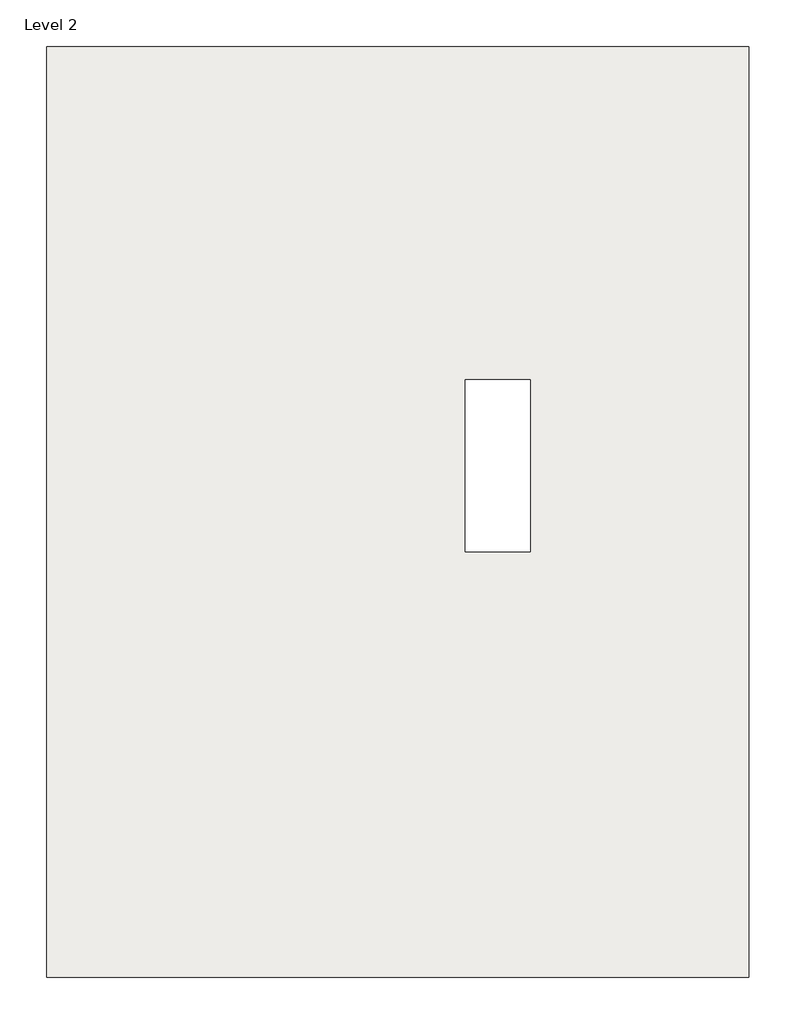
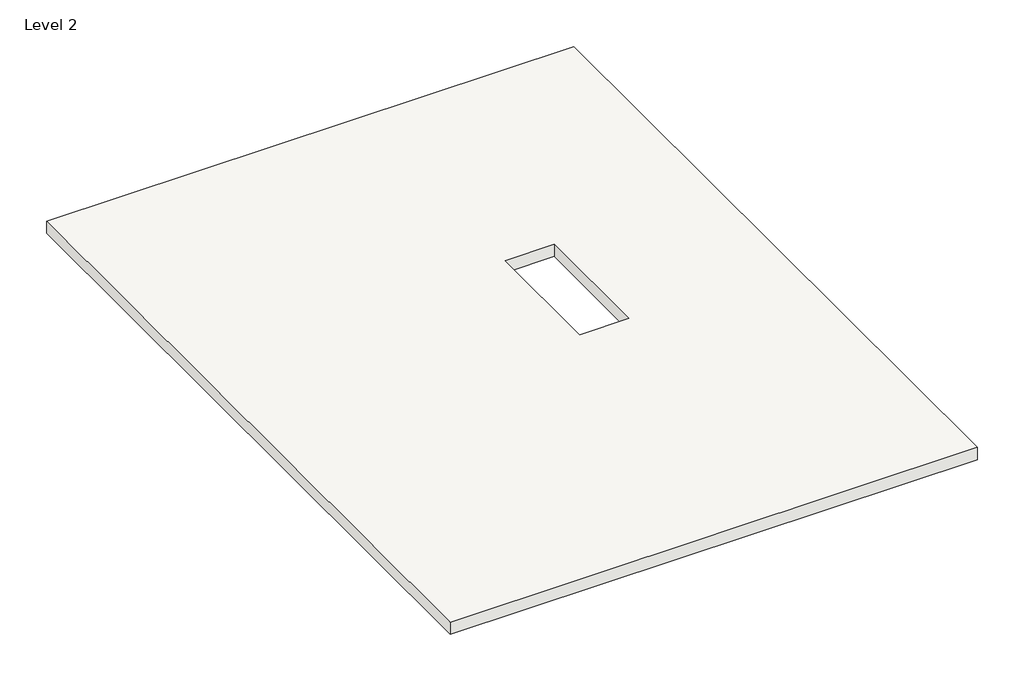
# One storey: 1 roof.
"""IFC4 building model written with IfcOpenShell, lengths in millimetres."""

from ifc_helpers import new_model, si_unit, frame, origin, place, context, project, spatial, polyline, outline, extrude, element, save

model = new_model("IFC4")

# Units and contexts
model_context = context("Model", 3, world=origin())
ifc_project = project(units=[si_unit("LENGTHUNIT", "METRE", prefix="MILLI")], contexts=[model_context])

# Site, building, storey
site = spatial("IfcSite", under=ifc_project)
building = spatial("IfcBuilding", under=site)
storey = spatial("IfcBuildingStorey", under=building, Name="Level 2", Elevation=3048.0)

# Roof
placement = place(None, origin())
element("IfcRoof", 1, ObjectType="Generic - 12\"", at=placement, inside=storey, context=model_context, shape_type="SweptSolid", body=[
    extrude(outline(polyline([(-11137.7350785, 11687.1033005), (1435.2649215, 11687.1033005), (1435.2649215, -4975.2966995), (-11137.7350785, -4975.2966995), (-11137.7350785, 11687.1033005)]), holes=[polyline([(-3644.7350785, 2644.7033005), (-2476.3350785, 2644.7033005), (-2476.3350785, 5724.4533005), (-3644.7350785, 5724.4533005), (-3644.7350785, 2644.7033005)])]), frame((0.0, 0.0, 3048.0), z_axis=(0.0, 0.0, 1.0), x_axis=(1.0, 0.0, 0.0)), (0.0, 0.0, 1.0), 304.8),
])

save(model, "model.ifc")

# Revit data of these elements
# Type "Generic - 12\""
#   Assembly Code = "B1020"
#   Layers, outside or top first: 1' - 0" "Brick, Soldier Course" (function 1)
# Element 1 (IfcRoof, "Generic - 12\"")
#   built-in parameter 1001705 = 11 (stored number, unit not read)
#   built-in parameter 1001710 = 33615
#   Phase Created = New Construction
#   Materials on its faces: "Brick, Soldier Course"
# Materials
#   "Brick, Soldier Course": class "Masonry", colour RGB 170 98 104, transparency 0, Description = "Common brick soldier coursed", Cost = 0
